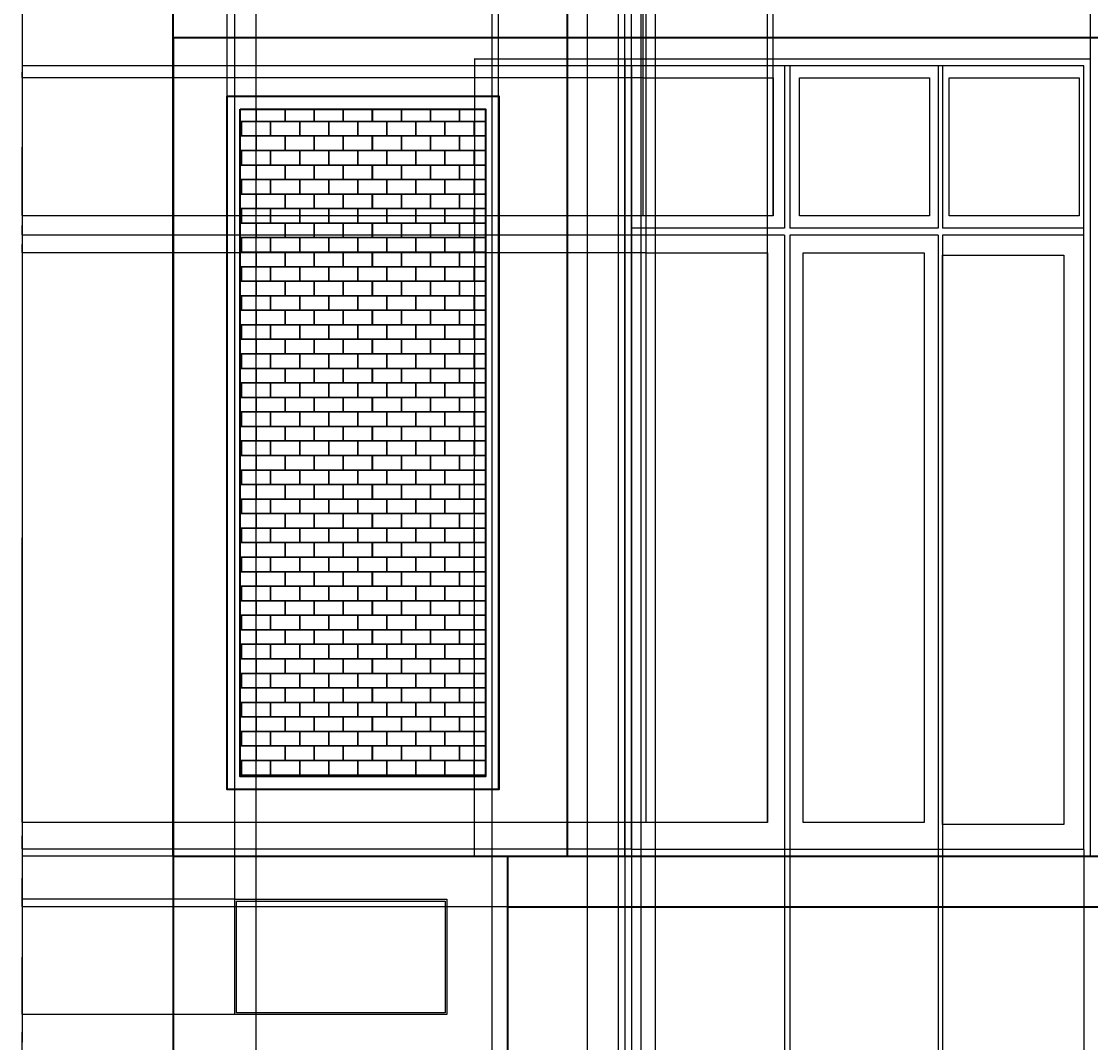
# Model space of a CAD drawing. Units: inches. Extents: x 1231 to 2151, y 481 to 2277.
# Tile 5 of 7: x 1231 to 1819, y 1373 to 1935. Entities that reach past the tile are written whole.
import ezdxf

# ---------------------------------------------------------------- set-up
doc = ezdxf.new("R2010")
doc.units = ezdxf.units.IN
doc.header["$MEASUREMENT"] = 0
for name, color, linetype, lineweight in [('A-ANNO-DIMS', 2, 'Continuous', 18), ('A-DOOR', 4, 'Continuous', 25), ('A-ELEV', 7, 'Continuous', 35), ('A-GLAZ', 3, 'Continuous', 25), ('A-WALL-PATT', 8, 'Continuous', 13)]:
    doc.layers.add(name, color=color, linetype=linetype, lineweight=lineweight)
doc.styles.get("Standard").update_dxf_attribs({"font": 'arial.ttf'})
doc.dimstyles.get("Standard").update_dxf_attribs({"dimtxt": 0.18, "dimasz": 0.18, "dimexe": 0.18, "dimexo": 0.0625, "dimgap": 0.09, "dimtad": 0, "dimtih": 1, "dimtoh": 1, "dimdec": 0, "dimzin": 0, "dimdsep": 46, "dimlunit": 3, "dimtxsty": 'Standard', "dimcen": 0.09, "dimadec": 0, "dimazin": 0, "dimtfac": 1, "dimtdec": 0, "dimtofl": 0, "dimtmove": 0, "dimatfit": 3, "dimfxl": 1, "dimtolj": 1, "dimtzin": 0, "dimarcsym": 0})

# ---------------------------------------------------------------- blocks, each defined once
blk = doc.blocks.new('*D2')
at = {"layer": 'A-ANNO-DIMS', "color": 0, "lineweight": -2, "transparency": 16777216}
for p, q in [((1314.18, 2193.78), (1230.78, 2193.78)), ((1230.96, 2193.6), (1230.96, 1378.92)), ((1230.96, 563.87), (1230.96, 1378.55)), ((1314.18, 563.69), (1230.78, 563.69))]:
    blk.add_line(p, q, dxfattribs=at)
at = {"layer": 'A-ANNO-DIMS', "color": 0, "transparency": 16777216}
for points in [[(1230.93, 2193.6), (1230.99, 2193.6), (1230.96, 2193.78)], [(1230.93, 563.87), (1230.99, 563.87), (1230.96, 563.69)]]:
    blk.add_solid(points, dxfattribs=at)
at = {"layer": 'Defpoints', "color": 0, "transparency": 16777216}
for p in [(1230.96, 2193.78), (1314.24, 2193.78), (1314.24, 563.69)]:
    blk.add_point(p, dxfattribs=at)
at = {"layer": 'A-ANNO-DIMS', "color": 0, "transparency": 16777216, "insert": (1230.96, 1378.74), "char_height": 0.18, "attachment_point": 5}
blk.add_mtext('\\A1;1630', dxfattribs=at)
blk = doc.blocks.new('*D15')
at = {"layer": 'A-ANNO-DIMS', "color": 0, "lineweight": -2, "transparency": 16777216}
for p, q in [((1314.24, 1475.61), (1314.24, 2276.71)), ((1314.42, 2276.53), (1328.56, 2276.53)), ((1343.64, 2276.53), (1329.49, 2276.53)), ((1343.82, 1512.24), (1343.82, 2276.71))]:
    blk.add_line(p, q, dxfattribs=at)
at = {"layer": 'A-ANNO-DIMS', "color": 0, "transparency": 16777216}
for points in [[(1314.42, 2276.56), (1314.42, 2276.5), (1314.24, 2276.53)], [(1343.64, 2276.56), (1343.64, 2276.5), (1343.82, 2276.53)]]:
    blk.add_solid(points, dxfattribs=at)
at = {"layer": 'Defpoints', "color": 0, "transparency": 16777216}
for p in [(1343.82, 2276.53), (1343.82, 1512.17), (1314.24, 1475.54)]:
    blk.add_point(p, dxfattribs=at)
at = {"layer": 'A-ANNO-DIMS', "color": 0, "transparency": 16777216, "insert": (1329.03, 2276.53), "char_height": 0.18, "attachment_point": 5}
blk.add_mtext('\\A1;29.575', dxfattribs=at)
blk = doc.blocks.new('*D16')
at = {"layer": 'A-ANNO-DIMS', "color": 0, "lineweight": -2, "transparency": 16777216}
for p, q in [((1343.82, 1512.24), (1343.82, 2276.71)), ((1344, 2276.53), (1418.14, 2276.53)), ((1493.2, 2276.53), (1419.06, 2276.53)), ((1493.38, 1512.24), (1493.38, 2276.71))]:
    blk.add_line(p, q, dxfattribs=at)
at = {"layer": 'A-ANNO-DIMS', "color": 0, "transparency": 16777216}
for points in [[(1344, 2276.56), (1344, 2276.5), (1343.82, 2276.53)], [(1493.2, 2276.56), (1493.2, 2276.5), (1493.38, 2276.53)]]:
    blk.add_solid(points, dxfattribs=at)
at = {"layer": 'Defpoints', "color": 0, "transparency": 16777216}
for p in [(1493.38, 2276.53), (1343.82, 1512.17), (1493.38, 1512.17)]:
    blk.add_point(p, dxfattribs=at)
at = {"layer": 'A-ANNO-DIMS', "color": 0, "transparency": 16777216, "insert": (1418.6, 2276.53), "char_height": 0.18, "attachment_point": 5}
blk.add_mtext('\\A1;149.57', dxfattribs=at)
blk = doc.blocks.new('*D17')
at = {"layer": 'A-ANNO-DIMS', "color": 0, "lineweight": -2, "transparency": 16777216}
for p, q in [((1493.38, 1512.24), (1493.38, 2276.71)), ((1493.56, 2276.53), (1527.71, 2276.53)), ((1562.61, 2276.53), (1528.46, 2276.53)), ((1562.79, 1475.61), (1562.79, 2276.71))]:
    blk.add_line(p, q, dxfattribs=at)
at = {"layer": 'A-ANNO-DIMS', "color": 0, "transparency": 16777216}
for points in [[(1493.56, 2276.56), (1493.56, 2276.5), (1493.38, 2276.53)], [(1562.61, 2276.56), (1562.61, 2276.5), (1562.79, 2276.53)]]:
    blk.add_solid(points, dxfattribs=at)
at = {"layer": 'Defpoints', "color": 0, "transparency": 16777216}
for p in [(1562.79, 2276.53), (1493.38, 1512.17), (1562.79, 1475.54)]:
    blk.add_point(p, dxfattribs=at)
at = {"layer": 'A-ANNO-DIMS', "color": 0, "transparency": 16777216, "insert": (1528.09, 2276.53), "char_height": 0.18, "attachment_point": 5}
blk.add_mtext('\\A1;69.41', dxfattribs=at)
blk = doc.blocks.new('*D18')
at = {"layer": 'A-ANNO-DIMS', "color": 0, "lineweight": -2, "transparency": 16777216}
for p, q in [((1562.79, 1914.62), (1562.79, 2276.71)), ((1562.97, 2276.53), (1690.65, 2276.53)), ((1819.13, 2276.53), (1691.45, 2276.53)), ((1819.31, 1914.62), (1819.31, 2276.71))]:
    blk.add_line(p, q, dxfattribs=at)
at = {"layer": 'A-ANNO-DIMS', "color": 0, "transparency": 16777216}
for points in [[(1562.97, 2276.56), (1562.97, 2276.5), (1562.79, 2276.53)], [(1819.13, 2276.56), (1819.13, 2276.5), (1819.31, 2276.53)]]:
    blk.add_solid(points, dxfattribs=at)
at = {"layer": 'Defpoints', "color": 0, "transparency": 16777216}
for p in [(1819.31, 2276.53), (1562.79, 1914.56), (1819.31, 1914.56)]:
    blk.add_point(p, dxfattribs=at)
at = {"layer": 'A-ANNO-DIMS', "color": 0, "transparency": 16777216, "insert": (1691.05, 2276.53), "char_height": 0.18, "attachment_point": 5}
blk.add_mtext('\\A1;256.5', dxfattribs=at)
blk = doc.blocks.new('*D32')
at = {"layer": 'A-ANNO-DIMS', "color": 0, "lineweight": -2, "transparency": 16777216}
for p, q in [((1314.24, 1043.75), (1314.24, 2276.71)), ((1314.42, 2276.53), (1336.68, 2276.53)), ((1359.73, 2276.53), (1337.47, 2276.53)), ((1359.91, 1037.75), (1359.91, 2276.71))]:
    blk.add_line(p, q, dxfattribs=at)
at = {"layer": 'A-ANNO-DIMS', "color": 0, "transparency": 16777216}
for points in [[(1314.42, 2276.56), (1314.42, 2276.5), (1314.24, 2276.53)], [(1359.73, 2276.56), (1359.73, 2276.5), (1359.91, 2276.53)]]:
    blk.add_solid(points, dxfattribs=at)
at = {"layer": 'Defpoints', "color": 0, "transparency": 16777216}
for p in [(1359.91, 2276.53), (1314.24, 1043.69), (1359.91, 1037.69)]:
    blk.add_point(p, dxfattribs=at)
at = {"layer": 'A-ANNO-DIMS', "color": 0, "transparency": 16777216, "insert": (1337.07, 2276.53), "char_height": 0.18, "attachment_point": 5}
blk.add_mtext('\\A1;45.67', dxfattribs=at)
blk = doc.blocks.new('*D33')
at = {"layer": 'A-ANNO-DIMS', "color": 0, "lineweight": -2, "transparency": 16777216}
for p, q in [((1359.91, 1037.75), (1359.91, 2276.71)), ((1360.09, 2276.53), (1424.43, 2276.53)), ((1489.68, 2276.53), (1425.34, 2276.53)), ((1489.86, 1037.75), (1489.86, 2276.71))]:
    blk.add_line(p, q, dxfattribs=at)
at = {"layer": 'A-ANNO-DIMS', "color": 0, "transparency": 16777216}
for points in [[(1360.09, 2276.56), (1360.09, 2276.5), (1359.91, 2276.53)], [(1489.68, 2276.56), (1489.68, 2276.5), (1489.86, 2276.53)]]:
    blk.add_solid(points, dxfattribs=at)
at = {"layer": 'Defpoints', "color": 0, "transparency": 16777216}
for p in [(1489.86, 2276.53), (1359.91, 1037.69), (1489.86, 1037.69)]:
    blk.add_point(p, dxfattribs=at)
at = {"layer": 'A-ANNO-DIMS', "color": 0, "transparency": 16777216, "insert": (1424.88, 2276.53), "char_height": 0.18, "attachment_point": 5}
blk.add_mtext('\\A1;129.95', dxfattribs=at)
blk = doc.blocks.new('*D34')
at = {"layer": 'A-ANNO-DIMS', "color": 0, "lineweight": -2, "transparency": 16777216}
for p, q in [((1489.86, 1037.75), (1489.86, 2276.71)), ((1490.04, 2276.53), (1515.72, 2276.53)), ((1542.2, 2276.53), (1516.51, 2276.53)), ((1542.38, 1043.75), (1542.38, 2276.71))]:
    blk.add_line(p, q, dxfattribs=at)
at = {"layer": 'A-ANNO-DIMS', "color": 0, "transparency": 16777216}
for points in [[(1490.04, 2276.56), (1490.04, 2276.5), (1489.86, 2276.53)], [(1542.2, 2276.56), (1542.2, 2276.5), (1542.38, 2276.53)]]:
    blk.add_solid(points, dxfattribs=at)
at = {"layer": 'Defpoints', "color": 0, "transparency": 16777216}
for p in [(1542.38, 2276.53), (1542.38, 1043.69), (1489.86, 1037.69)]:
    blk.add_point(p, dxfattribs=at)
at = {"layer": 'A-ANNO-DIMS', "color": 0, "transparency": 16777216, "insert": (1516.12, 2276.53), "char_height": 0.18, "attachment_point": 5}
blk.add_mtext('\\A1;52.52', dxfattribs=at)
blk = doc.blocks.new('*D35')
at = {"layer": 'A-ANNO-DIMS', "color": 0, "lineweight": -2, "transparency": 16777216}
for p, q in [((1542.38, 1043.75), (1542.38, 2276.71)), ((1542.56, 2276.53), (1556.6, 2276.53)), ((1571.58, 2276.53), (1557.53, 2276.53)), ((1571.76, 1043.75), (1571.76, 2276.71))]:
    blk.add_line(p, q, dxfattribs=at)
at = {"layer": 'A-ANNO-DIMS', "color": 0, "transparency": 16777216}
for points in [[(1542.56, 2276.56), (1542.56, 2276.5), (1542.38, 2276.53)], [(1571.58, 2276.56), (1571.58, 2276.5), (1571.76, 2276.53)]]:
    blk.add_solid(points, dxfattribs=at)
at = {"layer": 'Defpoints', "color": 0, "transparency": 16777216}
for p in [(1571.76, 2276.53), (1542.38, 1043.69), (1571.76, 1043.69)]:
    blk.add_point(p, dxfattribs=at)
at = {"layer": 'A-ANNO-DIMS', "color": 0, "transparency": 16777216, "insert": (1557.07, 2276.53), "char_height": 0.18, "attachment_point": 5}
blk.add_mtext('\\A1;29.385', dxfattribs=at)
blk = doc.blocks.new('*D36')
at = {"layer": 'A-ANNO-DIMS', "color": 0, "lineweight": -2, "transparency": 16777216}
for p, q in [((1571.76, 1043.75), (1571.76, 2276.71)), ((1571.94, 2276.53), (1575.38, 2276.53)), ((1579.61, 2276.53), (1576.17, 2276.53)), ((1579.79, 1032.87), (1579.79, 2276.71))]:
    blk.add_line(p, q, dxfattribs=at)
at = {"layer": 'A-ANNO-DIMS', "color": 0, "transparency": 16777216}
for points in [[(1571.94, 2276.56), (1571.94, 2276.5), (1571.76, 2276.53)], [(1579.61, 2276.56), (1579.61, 2276.5), (1579.79, 2276.53)]]:
    blk.add_solid(points, dxfattribs=at)
at = {"layer": 'Defpoints', "color": 0, "transparency": 16777216}
for p in [(1579.79, 2276.53), (1571.76, 1043.69), (1579.79, 1032.81)]:
    blk.add_point(p, dxfattribs=at)
at = {"layer": 'A-ANNO-DIMS', "color": 0, "transparency": 16777216, "insert": (1575.78, 2276.53), "char_height": 0.18, "attachment_point": 5}
blk.add_mtext('\\A1;8.033', dxfattribs=at)
blk = doc.blocks.new('*D50')
at = {"layer": 'A-ANNO-DIMS', "color": 0, "lineweight": -2, "transparency": 16777216}
for p, q in [((1542.38, 563.75), (1542.38, 2276.71)), ((1542.56, 2276.53), (1550.52, 2276.53)), ((1559.26, 2276.53), (1551.3, 2276.53)), ((1559.44, 576.65), (1559.44, 2276.71))]:
    blk.add_line(p, q, dxfattribs=at)
at = {"layer": 'A-ANNO-DIMS', "color": 0, "transparency": 16777216}
for points in [[(1542.56, 2276.56), (1542.56, 2276.5), (1542.38, 2276.53)], [(1559.26, 2276.56), (1559.26, 2276.5), (1559.44, 2276.53)]]:
    blk.add_solid(points, dxfattribs=at)
at = {"layer": 'Defpoints', "color": 0, "transparency": 16777216}
for p in [(1559.44, 2276.53), (1559.44, 576.59), (1542.38, 563.69)]:
    blk.add_point(p, dxfattribs=at)
at = {"layer": 'A-ANNO-DIMS', "color": 0, "transparency": 16777216, "insert": (1550.91, 2276.53), "char_height": 0.18, "attachment_point": 5}
blk.add_mtext('\\A1;17.07', dxfattribs=at)
blk = doc.blocks.new('*D58')
at = {"layer": 'A-ANNO-DIMS', "color": 0, "lineweight": -2, "transparency": 16777216}
for p, q in [((1314.24, 1475.61), (1314.24, 2276.71)), ((1314.42, 2276.53), (1330.74, 2276.53)), ((1347.85, 2276.53), (1331.53, 2276.53)), ((1348.03, 1451.84), (1348.03, 2276.71))]:
    blk.add_line(p, q, dxfattribs=at)
at = {"layer": 'A-ANNO-DIMS', "color": 0, "transparency": 16777216}
for points in [[(1314.42, 2276.56), (1314.42, 2276.5), (1314.24, 2276.53)], [(1347.85, 2276.56), (1347.85, 2276.5), (1348.03, 2276.53)]]:
    blk.add_solid(points, dxfattribs=at)
at = {"layer": 'Defpoints', "color": 0, "transparency": 16777216}
for p in [(1348.03, 2276.53), (1314.24, 1475.54), (1348.03, 1451.77)]:
    blk.add_point(p, dxfattribs=at)
at = {"layer": 'A-ANNO-DIMS', "color": 0, "transparency": 16777216, "insert": (1331.14, 2276.53), "char_height": 0.18, "attachment_point": 5}
blk.add_mtext('\\A1;33.79', dxfattribs=at)
blk = doc.blocks.new('*D59')
at = {"layer": 'A-ANNO-DIMS', "color": 0, "lineweight": -2, "transparency": 16777216}
for p, q in [((1314.18, 1475.54), (1230.78, 1475.54)), ((1230.96, 1475.36), (1230.96, 1463.84)), ((1230.96, 1451.95), (1230.96, 1463.48)), ((1347.97, 1451.77), (1230.78, 1451.77))]:
    blk.add_line(p, q, dxfattribs=at)
at = {"layer": 'A-ANNO-DIMS', "color": 0, "transparency": 16777216}
for points in [[(1230.93, 1475.36), (1230.99, 1475.36), (1230.96, 1475.54)], [(1230.93, 1451.95), (1230.99, 1451.95), (1230.96, 1451.77)]]:
    blk.add_solid(points, dxfattribs=at)
at = {"layer": 'Defpoints', "color": 0, "transparency": 16777216}
for p in [(1314.24, 1475.54), (1230.96, 1451.77), (1348.03, 1451.77)]:
    blk.add_point(p, dxfattribs=at)
at = {"layer": 'A-ANNO-DIMS', "color": 0, "transparency": 16777216, "insert": (1230.96, 1463.66), "char_height": 0.18, "attachment_point": 5}
blk.add_mtext('\\A1;23.77', dxfattribs=at)
blk = doc.blocks.new('*D60')
at = {"layer": 'A-ANNO-DIMS', "color": 0, "lineweight": -2, "transparency": 16777216}
for p, q in [((1347.97, 1451.77), (1230.78, 1451.77)), ((1230.96, 1451.59), (1230.96, 1420.21)), ((1230.96, 1388.46), (1230.96, 1419.84)), ((1347.97, 1388.28), (1230.78, 1388.28))]:
    blk.add_line(p, q, dxfattribs=at)
at = {"layer": 'A-ANNO-DIMS', "color": 0, "transparency": 16777216}
for points in [[(1230.93, 1451.59), (1230.99, 1451.59), (1230.96, 1451.77)], [(1230.93, 1388.46), (1230.99, 1388.46), (1230.96, 1388.28)]]:
    blk.add_solid(points, dxfattribs=at)
at = {"layer": 'Defpoints', "color": 0, "transparency": 16777216}
for p in [(1348.03, 1451.77), (1230.96, 1388.28), (1348.03, 1388.28)]:
    blk.add_point(p, dxfattribs=at)
at = {"layer": 'A-ANNO-DIMS', "color": 0, "transparency": 16777216, "insert": (1230.96, 1420.03), "char_height": 0.18, "attachment_point": 5}
blk.add_mtext('\\A1;63.5', dxfattribs=at)
blk = doc.blocks.new('*D61')
at = {"layer": 'A-ANNO-DIMS', "color": 0, "lineweight": -2, "transparency": 16777216}
for p, q in [((1347.97, 1388.28), (1230.78, 1388.28)), ((1230.96, 1388.1), (1230.96, 1372.98)), ((1230.96, 1357.51), (1230.96, 1372.62)), ((1347.97, 1357.33), (1230.78, 1357.33))]:
    blk.add_line(p, q, dxfattribs=at)
at = {"layer": 'A-ANNO-DIMS', "color": 0, "transparency": 16777216}
for points in [[(1230.93, 1388.1), (1230.99, 1388.1), (1230.96, 1388.28)], [(1230.93, 1357.51), (1230.99, 1357.51), (1230.96, 1357.33)]]:
    blk.add_solid(points, dxfattribs=at)
at = {"layer": 'Defpoints', "color": 0, "transparency": 16777216}
for p in [(1348.03, 1388.28), (1230.96, 1357.33), (1348.03, 1357.33)]:
    blk.add_point(p, dxfattribs=at)
at = {"layer": 'A-ANNO-DIMS', "color": 0, "transparency": 16777216, "insert": (1230.96, 1372.8), "char_height": 0.18, "attachment_point": 5}
blk.add_mtext('\\A1;30.954', dxfattribs=at)
blk = doc.blocks.new('*D67')
at = {"layer": 'A-ANNO-DIMS', "color": 0, "lineweight": -2, "transparency": 16777216}
for p, q in [((1498.25, 1475.54), (1230.78, 1475.54)), ((1230.96, 1475.36), (1230.96, 1461.72)), ((1230.96, 1447.72), (1230.96, 1461.36)), ((1498.25, 1447.54), (1230.78, 1447.54))]:
    blk.add_line(p, q, dxfattribs=at)
at = {"layer": 'A-ANNO-DIMS', "color": 0, "transparency": 16777216}
for points in [[(1230.93, 1475.36), (1230.99, 1475.36), (1230.96, 1475.54)], [(1230.93, 1447.72), (1230.99, 1447.72), (1230.96, 1447.54)]]:
    blk.add_solid(points, dxfattribs=at)
at = {"layer": 'Defpoints', "color": 0, "transparency": 16777216}
for p in [(1230.96, 1475.54), (1498.31, 1475.54), (1498.31, 1447.54)]:
    blk.add_point(p, dxfattribs=at)
at = {"layer": 'A-ANNO-DIMS', "color": 0, "transparency": 16777216, "insert": (1230.96, 1461.54), "char_height": 0.18, "attachment_point": 5}
blk.add_mtext('\\A1;28.005', dxfattribs=at)
blk = doc.blocks.new('*D83')
at = {"layer": 'A-ANNO-DIMS', "color": 0, "lineweight": -2, "transparency": 16777216}
for p, q in [((1562.73, 1914.56), (1479.86, 1914.56)), ((1480.04, 1914.38), (1480.04, 1695.23)), ((1480.04, 1475.72), (1480.04, 1694.87)), ((1562.73, 1475.54), (1479.86, 1475.54))]:
    blk.add_line(p, q, dxfattribs=at)
at = {"layer": 'A-ANNO-DIMS', "color": 0, "transparency": 16777216}
for points in [[(1480.01, 1914.38), (1480.07, 1914.38), (1480.04, 1914.56)], [(1480.01, 1475.72), (1480.07, 1475.72), (1480.04, 1475.54)]]:
    blk.add_solid(points, dxfattribs=at)
at = {"layer": 'Defpoints', "color": 0, "transparency": 16777216}
for p in [(1480.04, 1914.56), (1562.79, 1914.56), (1562.79, 1475.54)]:
    blk.add_point(p, dxfattribs=at)
at = {"layer": 'A-ANNO-DIMS', "color": 0, "transparency": 16777216, "insert": (1480.04, 1695.05), "char_height": 0.18, "attachment_point": 5}
blk.add_mtext('\\A1;439', dxfattribs=at)
blk = doc.blocks.new('*D84')
at = {"layer": 'A-ANNO-DIMS', "color": 0, "lineweight": -2, "transparency": 16777216}
for p, q in [((1574.54, 1494.13), (1230.78, 1494.13)), ((1230.96, 1493.95), (1230.96, 1486.91)), ((1230.96, 1479.5), (1230.96, 1486.54)), ((1566.5, 1479.32), (1230.78, 1479.32))]:
    blk.add_line(p, q, dxfattribs=at)
at = {"layer": 'A-ANNO-DIMS', "color": 0, "transparency": 16777216}
for points in [[(1230.93, 1493.95), (1230.99, 1493.95), (1230.96, 1494.13)], [(1230.93, 1479.5), (1230.99, 1479.5), (1230.96, 1479.32)]]:
    blk.add_solid(points, dxfattribs=at)
at = {"layer": 'Defpoints', "color": 0, "transparency": 16777216}
for p in [(1230.96, 1494.13), (1574.6, 1494.13), (1566.56, 1479.32)]:
    blk.add_point(p, dxfattribs=at)
at = {"layer": 'A-ANNO-DIMS', "color": 0, "transparency": 16777216, "insert": (1230.96, 1486.72), "char_height": 0.18, "attachment_point": 5}
blk.add_mtext('\\A1;14.818', dxfattribs=at)
blk = doc.blocks.new('*D85')
at = {"layer": 'A-ANNO-DIMS', "color": 0, "lineweight": -2, "transparency": 16777216}
for p, q in [((1574.54, 1807.75), (1230.78, 1807.75)), ((1230.96, 1807.57), (1230.96, 1651.12)), ((1230.96, 1494.31), (1230.96, 1650.76)), ((1574.54, 1494.13), (1230.78, 1494.13))]:
    blk.add_line(p, q, dxfattribs=at)
at = {"layer": 'A-ANNO-DIMS', "color": 0, "transparency": 16777216}
for points in [[(1230.93, 1807.57), (1230.99, 1807.57), (1230.96, 1807.75)], [(1230.93, 1494.31), (1230.99, 1494.31), (1230.96, 1494.13)]]:
    blk.add_solid(points, dxfattribs=at)
at = {"layer": 'Defpoints', "color": 0, "transparency": 16777216}
for p in [(1230.96, 1807.75), (1574.6, 1807.75), (1574.6, 1494.13)]:
    blk.add_point(p, dxfattribs=at)
at = {"layer": 'A-ANNO-DIMS', "color": 0, "transparency": 16777216, "insert": (1230.96, 1650.94), "char_height": 0.18, "attachment_point": 5}
blk.add_mtext('\\A1;313.6', dxfattribs=at)
blk = doc.blocks.new('*D86')
at = {"layer": 'A-ANNO-DIMS', "color": 0, "lineweight": -2, "transparency": 16777216}
for p, q in [((1566.5, 1817.51), (1230.78, 1817.51)), ((1230.96, 1817.33), (1230.96, 1812.81)), ((1574.54, 1807.75), (1230.78, 1807.75)), ((1230.96, 1807.93), (1230.96, 1812.45))]:
    blk.add_line(p, q, dxfattribs=at)
at = {"layer": 'A-ANNO-DIMS', "color": 0, "transparency": 16777216}
for points in [[(1230.93, 1817.33), (1230.99, 1817.33), (1230.96, 1817.51)], [(1230.93, 1807.93), (1230.99, 1807.93), (1230.96, 1807.75)]]:
    blk.add_solid(points, dxfattribs=at)
at = {"layer": 'Defpoints', "color": 0, "transparency": 16777216}
for p in [(1230.96, 1817.51), (1566.56, 1817.51), (1574.6, 1807.75)]:
    blk.add_point(p, dxfattribs=at)
at = {"layer": 'A-ANNO-DIMS', "color": 0, "transparency": 16777216, "insert": (1230.96, 1812.63), "char_height": 0.18, "attachment_point": 5}
blk.add_mtext('\\A1;9.758', dxfattribs=at)
blk = doc.blocks.new('*D87')
at = {"layer": 'A-ANNO-DIMS', "color": 0, "lineweight": -2, "transparency": 16777216}
for p, q in [((1572.8, 1828.25), (1230.78, 1828.25)), ((1230.96, 1828.07), (1230.96, 1823.06)), ((1230.96, 1817.69), (1230.96, 1822.7)), ((1566.5, 1817.51), (1230.78, 1817.51))]:
    blk.add_line(p, q, dxfattribs=at)
at = {"layer": 'A-ANNO-DIMS', "color": 0, "transparency": 16777216}
for points in [[(1230.93, 1828.07), (1230.99, 1828.07), (1230.96, 1828.25)], [(1230.93, 1817.69), (1230.99, 1817.69), (1230.96, 1817.51)]]:
    blk.add_solid(points, dxfattribs=at)
at = {"layer": 'Defpoints', "color": 0, "transparency": 16777216}
for p in [(1230.96, 1828.25), (1572.87, 1828.25), (1566.56, 1817.51)]:
    blk.add_point(p, dxfattribs=at)
at = {"layer": 'A-ANNO-DIMS', "color": 0, "transparency": 16777216, "insert": (1230.96, 1822.88), "char_height": 0.18, "attachment_point": 5}
blk.add_mtext('\\A1;10.739', dxfattribs=at)
blk = doc.blocks.new('*D88')
at = {"layer": 'A-ANNO-DIMS', "color": 0, "lineweight": -2, "transparency": 16777216}
for p, q in [((1572.8, 1904.15), (1230.78, 1904.15)), ((1230.96, 1903.97), (1230.96, 1866.38)), ((1230.96, 1828.43), (1230.96, 1866.02)), ((1572.8, 1828.25), (1230.78, 1828.25))]:
    blk.add_line(p, q, dxfattribs=at)
at = {"layer": 'A-ANNO-DIMS', "color": 0, "transparency": 16777216}
for points in [[(1230.93, 1903.97), (1230.99, 1903.97), (1230.96, 1904.15)], [(1230.93, 1828.43), (1230.99, 1828.43), (1230.96, 1828.25)]]:
    blk.add_solid(points, dxfattribs=at)
at = {"layer": 'Defpoints', "color": 0, "transparency": 16777216}
for p in [(1230.96, 1904.15), (1572.87, 1904.15), (1572.87, 1828.25)]:
    blk.add_point(p, dxfattribs=at)
at = {"layer": 'A-ANNO-DIMS', "color": 0, "transparency": 16777216, "insert": (1230.96, 1866.2), "char_height": 0.18, "attachment_point": 5}
blk.add_mtext('\\A1;75.9', dxfattribs=at)
blk = doc.blocks.new('*D89')
at = {"layer": 'A-ANNO-DIMS', "color": 0, "lineweight": -2, "transparency": 16777216}
for p, q in [((1566.5, 1910.79), (1230.78, 1910.79)), ((1230.96, 1910.61), (1230.96, 1907.65)), ((1572.8, 1904.15), (1230.78, 1904.15)), ((1230.96, 1904.33), (1230.96, 1907.28))]:
    blk.add_line(p, q, dxfattribs=at)
at = {"layer": 'A-ANNO-DIMS', "color": 0, "transparency": 16777216}
for points in [[(1230.93, 1910.61), (1230.99, 1910.61), (1230.96, 1910.79)], [(1230.93, 1904.33), (1230.99, 1904.33), (1230.96, 1904.15)]]:
    blk.add_solid(points, dxfattribs=at)
at = {"layer": 'Defpoints', "color": 0, "transparency": 16777216}
for p in [(1230.96, 1910.79), (1566.56, 1910.79), (1572.87, 1904.15)]:
    blk.add_point(p, dxfattribs=at)
at = {"layer": 'A-ANNO-DIMS', "color": 0, "transparency": 16777216, "insert": (1230.96, 1907.47), "char_height": 0.18, "attachment_point": 5}
blk.add_mtext('\\A1;6.64', dxfattribs=at)
blk = doc.blocks.new('*D90')
at = {"layer": 'A-ANNO-DIMS', "color": 0, "lineweight": -2, "transparency": 16777216}
for p, q in [((1566.56, 1479.25), (1566.56, 480.76)), ((1562.79, 1475.48), (1562.79, 480.76)), ((1562.97, 480.94), (1564.3, 480.94)), ((1566.38, 480.94), (1565.05, 480.94))]:
    blk.add_line(p, q, dxfattribs=at)
at = {"layer": 'A-ANNO-DIMS', "color": 0, "transparency": 16777216}
for points in [[(1562.97, 480.97), (1562.97, 480.91), (1562.79, 480.94)], [(1566.38, 480.97), (1566.38, 480.91), (1566.56, 480.94)]]:
    blk.add_solid(points, dxfattribs=at)
at = {"layer": 'Defpoints', "color": 0, "transparency": 16777216}
for p in [(1566.56, 1479.32), (1562.79, 1475.54), (1566.56, 480.94)]:
    blk.add_point(p, dxfattribs=at)
at = {"layer": 'A-ANNO-DIMS', "color": 0, "transparency": 16777216, "insert": (1564.68, 480.94), "char_height": 0.18, "attachment_point": 5}
blk.add_mtext('\\A1;3.771', dxfattribs=at)
blk = doc.blocks.new('*D91')
at = {"layer": 'A-ANNO-DIMS', "color": 0, "lineweight": -2, "transparency": 16777216}
for p, q in [((1566.56, 1479.25), (1566.56, 480.76)), ((1650.77, 1479.25), (1650.77, 480.76)), ((1566.74, 480.94), (1608.34, 480.94)), ((1650.59, 480.94), (1608.99, 480.94))]:
    blk.add_line(p, q, dxfattribs=at)
at = {"layer": 'A-ANNO-DIMS', "color": 0, "transparency": 16777216}
for points in [[(1566.74, 480.97), (1566.74, 480.91), (1566.56, 480.94)], [(1650.59, 480.97), (1650.59, 480.91), (1650.77, 480.94)]]:
    blk.add_solid(points, dxfattribs=at)
at = {"layer": 'Defpoints', "color": 0, "transparency": 16777216}
for p in [(1566.56, 1479.32), (1650.77, 1479.32), (1650.77, 480.94)]:
    blk.add_point(p, dxfattribs=at)
at = {"layer": 'A-ANNO-DIMS', "color": 0, "transparency": 16777216, "insert": (1608.66, 480.94), "char_height": 0.18, "attachment_point": 5}
blk.add_mtext('\\A1;84.2', dxfattribs=at)
blk = doc.blocks.new('*D92')
at = {"layer": 'A-ANNO-DIMS', "color": 0, "lineweight": -2, "transparency": 16777216}
for p, q in [((1653.67, 1479.25), (1653.67, 480.76)), ((1735.42, 1479.25), (1735.42, 480.76)), ((1653.85, 480.94), (1694.15, 480.94)), ((1735.24, 480.94), (1694.94, 480.94))]:
    blk.add_line(p, q, dxfattribs=at)
at = {"layer": 'A-ANNO-DIMS', "color": 0, "transparency": 16777216}
for points in [[(1653.85, 480.97), (1653.85, 480.91), (1653.67, 480.94)], [(1735.24, 480.97), (1735.24, 480.91), (1735.42, 480.94)]]:
    blk.add_solid(points, dxfattribs=at)
at = {"layer": 'Defpoints', "color": 0, "transparency": 16777216}
for p in [(1653.67, 1479.32), (1735.42, 1479.32), (1735.42, 480.94)]:
    blk.add_point(p, dxfattribs=at)
at = {"layer": 'A-ANNO-DIMS', "color": 0, "transparency": 16777216, "insert": (1694.55, 480.94), "char_height": 0.18, "attachment_point": 5}
blk.add_mtext('\\A1;81.75', dxfattribs=at)
blk = doc.blocks.new('*D93')
at = {"layer": 'A-ANNO-DIMS', "color": 0, "lineweight": -2, "transparency": 16777216}
for p, q in [((1737.75, 1479.25), (1737.75, 480.76)), ((1815.54, 1479.25), (1815.54, 480.76)), ((1737.93, 480.94), (1776.25, 480.94)), ((1815.36, 480.94), (1777.04, 480.94))]:
    blk.add_line(p, q, dxfattribs=at)
at = {"layer": 'A-ANNO-DIMS', "color": 0, "transparency": 16777216}
for points in [[(1737.93, 480.97), (1737.93, 480.91), (1737.75, 480.94)], [(1815.36, 480.97), (1815.36, 480.91), (1815.54, 480.94)]]:
    blk.add_solid(points, dxfattribs=at)
at = {"layer": 'Defpoints', "color": 0, "transparency": 16777216}
for p in [(1737.75, 1479.32), (1815.54, 1479.32), (1815.54, 480.94)]:
    blk.add_point(p, dxfattribs=at)
at = {"layer": 'A-ANNO-DIMS', "color": 0, "transparency": 16777216, "insert": (1776.64, 480.94), "char_height": 0.18, "attachment_point": 5}
blk.add_mtext('\\A1;77.79', dxfattribs=at)
blk = doc.blocks.new('*D94')
at = {"layer": 'A-ANNO-DIMS', "color": 0, "lineweight": -2, "transparency": 16777216}
for p, q in [((1566.56, 1479.38), (1566.56, 2276.71)), ((1566.74, 2276.53), (1570.19, 2276.53)), ((1574.42, 2276.53), (1570.98, 2276.53)), ((1574.6, 1494.2), (1574.6, 2276.71))]:
    blk.add_line(p, q, dxfattribs=at)
at = {"layer": 'A-ANNO-DIMS', "color": 0, "transparency": 16777216}
for points in [[(1566.74, 2276.56), (1566.74, 2276.5), (1566.56, 2276.53)], [(1574.42, 2276.56), (1574.42, 2276.5), (1574.6, 2276.53)]]:
    blk.add_solid(points, dxfattribs=at)
at = {"layer": 'Defpoints', "color": 0, "transparency": 16777216}
for p in [(1574.6, 2276.53), (1574.6, 1494.13), (1566.56, 1479.32)]:
    blk.add_point(p, dxfattribs=at)
at = {"layer": 'A-ANNO-DIMS', "color": 0, "transparency": 16777216, "insert": (1570.58, 2276.53), "char_height": 0.18, "attachment_point": 5}
blk.add_mtext('\\A1;8.042', dxfattribs=at)
blk = doc.blocks.new('*D95')
at = {"layer": 'A-ANNO-DIMS', "color": 0, "lineweight": -2, "transparency": 16777216}
for p, q in [((1574.6, 1494.2), (1574.6, 2276.71)), ((1574.78, 2276.53), (1607.58, 2276.53)), ((1641.16, 2276.53), (1608.37, 2276.53)), ((1641.34, 1494.2), (1641.34, 2276.71))]:
    blk.add_line(p, q, dxfattribs=at)
at = {"layer": 'A-ANNO-DIMS', "color": 0, "transparency": 16777216}
for points in [[(1574.78, 2276.56), (1574.78, 2276.5), (1574.6, 2276.53)], [(1641.16, 2276.56), (1641.16, 2276.5), (1641.34, 2276.53)]]:
    blk.add_solid(points, dxfattribs=at)
at = {"layer": 'Defpoints', "color": 0, "transparency": 16777216}
for p in [(1641.34, 2276.53), (1574.6, 1494.13), (1641.34, 1494.13)]:
    blk.add_point(p, dxfattribs=at)
at = {"layer": 'A-ANNO-DIMS', "color": 0, "transparency": 16777216, "insert": (1607.97, 2276.53), "char_height": 0.18, "attachment_point": 5}
blk.add_mtext('\\A1;66.74', dxfattribs=at)
blk = doc.blocks.new('*D96')
at = {"layer": 'A-ANNO-DIMS', "color": 0, "lineweight": -2, "transparency": 16777216}
for p, q in [((1572.87, 1828.31), (1572.87, 2276.71)), ((1573.05, 2276.53), (1608.26, 2276.53)), ((1644.26, 2276.53), (1609.05, 2276.53)), ((1644.44, 1828.31), (1644.44, 2276.71))]:
    blk.add_line(p, q, dxfattribs=at)
at = {"layer": 'A-ANNO-DIMS', "color": 0, "transparency": 16777216}
for points in [[(1573.05, 2276.56), (1573.05, 2276.5), (1572.87, 2276.53)], [(1644.26, 2276.56), (1644.26, 2276.5), (1644.44, 2276.53)]]:
    blk.add_solid(points, dxfattribs=at)
at = {"layer": 'Defpoints', "color": 0, "transparency": 16777216}
for p in [(1644.44, 2276.53), (1572.87, 1828.25), (1644.44, 1828.25)]:
    blk.add_point(p, dxfattribs=at)
at = {"layer": 'A-ANNO-DIMS', "color": 0, "transparency": 16777216, "insert": (1608.65, 2276.53), "char_height": 0.18, "attachment_point": 5}
blk.add_mtext('\\A1;71.57', dxfattribs=at)

msp = doc.modelspace()

# ---------------------------------------------------------------- hatches: boundary and pattern name
at = {"layer": 'A-WALL-PATT'}
h = msp.add_hatch(dxfattribs=at)
h.set_pattern_fill('AR-B816C', color=256)
h.paths.add_polyline_path([(1486.2072, 1886.877), (1350.9925, 1886.877), (1350.9925, 1519.3518), (1486.2072, 1519.3518)])

# ---------------------------------------------------------------- linework, layer by layer
at = {"layer": 'A-DOOR'}
for p, q in [((1819.3087, 1914.557), (1562.7916, 1914.557)), ((1562.7916, 1914.557), (1562.7916, 1475.5441)), ((1819.3087, 1475.5441), (1819.3087, 1914.557)), ((1815.5376, 1910.786), (1566.5626, 1910.786)), ((1566.5626, 1910.786), (1566.5626, 1479.3152)), ((1650.766, 1910.786), (1650.766, 1821.4896)), ((1653.6719, 1910.786), (1653.6719, 1821.4896)), ((1735.4237, 1910.786), (1735.4237, 1821.4896)), ((1737.7463, 1910.786), (1737.7463, 1821.4896)), ((1815.5376, 1479.3152), (1815.5376, 1910.786)), ((1650.766, 1821.4896), (1566.5626, 1821.4896)), ((1735.4237, 1821.4896), (1653.6719, 1821.4896)), ((1815.5376, 1821.4896), (1737.7463, 1821.4896)), ((1650.766, 1817.5102), (1566.5626, 1817.5102)), ((1650.766, 1817.5102), (1650.766, 1479.3152)), ((1653.6719, 1817.5102), (1653.6719, 1479.3152)), ((1735.4237, 1817.5102), (1653.6719, 1817.5102)), ((1735.4237, 1817.5102), (1735.4237, 1479.3152)), ((1815.5376, 1817.5102), (1737.7463, 1817.5102)), ((1737.7463, 1817.5102), (1737.7463, 1479.3152)), ((1566.5626, 1479.3152), (1815.5376, 1479.3152)), ((1562.7916, 1475.5441), (1819.3087, 1475.5441))]:
    msp.add_line(p, q, dxfattribs=at)
for points in [[(1572.8669, 1904.1464), (1644.4374, 1904.1464), (1644.4374, 1828.2487), (1572.8669, 1828.2487)], [(1659.0358, 1904.1464), (1730.6063, 1904.1464), (1730.6063, 1828.2487), (1659.0358, 1828.2487)], [(1741.4582, 1904.1464), (1813.0288, 1904.1464), (1813.0288, 1828.2487), (1741.4582, 1828.2487)], [(1574.6049, 1807.7526), (1641.3412, 1807.7526), (1641.3412, 1494.1329), (1574.6049, 1494.1329)], [(1660.9962, 1807.7526), (1727.7324, 1807.7526), (1727.7324, 1494.1329), (1660.9962, 1494.1329)], [(1737.7463, 1806.5252), (1804.4825, 1806.5252), (1804.4825, 1492.9055), (1737.7463, 1492.9055)]]:
    msp.add_lwpolyline(points, close=True, dxfattribs=at)
at = {"layer": 'A-ELEV'}
for p, q in [((1314.2408, 1475.5441), (1314.2408, 2193.7789)), ((1531.2103, 1475.5441), (1531.2103, 1973.8854)), ((2067.6855, 1926.2862), (1314.2408, 1926.2862)), ((1314.2408, 1926.2862), (1314.2408, 563.6912)), ((1314.2408, 1475.5441), (2067.6855, 1475.5441)), ((1498.3132, 1475.5441), (1498.3132, 1170.3351)), ((1498.3132, 1447.5396), (2067.6855, 1447.5396))]:
    msp.add_line(p, q, dxfattribs=at)
for points in [[(1343.8157, 1894.0538), (1493.3841, 1894.0538), (1493.3841, 1512.1749), (1343.8157, 1512.1749)], [(1350.9925, 1886.877), (1486.2072, 1886.877), (1486.2072, 1519.3518), (1350.9925, 1519.3518)]]:
    msp.add_lwpolyline(points, close=True, dxfattribs=at)
at = {"layer": 'A-GLAZ'}
for points in [[(1348.0309, 1451.7741), (1464.8184, 1451.7741), (1464.8184, 1388.2789), (1348.0309, 1388.2789)], [(1348.9993, 1450.8057), (1463.8499, 1450.8057), (1463.8499, 1389.2474), (1348.9993, 1389.2474)]]:
    msp.add_lwpolyline(points, close=True, dxfattribs=at)

# ---------------------------------------------------------------- dimensions: what is measured, and where the dimension line sits
at = {"layer": 'A-ANNO-DIMS'}
for base, p1, p2, override, picture, middle in [((1343.8157, 2276.5289), (1314.2408, 1475.5441), (1343.8157, 1512.1749), {"dimdec": 3, "dimlfac": 1, "dimrnd": 0, "dimzin": 0, "dimdsep": 46, "dimlunit": 2}, '*D15', (1329.0282, 2276.5289)), ((1359.9075, 2276.5289), (1314.2408, 1043.6912), (1359.9075, 1037.6872), {"dimdec": 2, "dimlfac": 1, "dimrnd": 0, "dimzin": 0, "dimdsep": 46, "dimlunit": 2}, '*D32', (1337.0741, 2276.5289)), ((1348.0309, 2276.5289), (1314.2408, 1475.5441), (1348.0309, 1451.7741), {"dimdec": 2, "dimlfac": 1, "dimrnd": 0, "dimzin": 0, "dimdsep": 46, "dimlunit": 2}, '*D58', (1331.1358, 2276.5289)), ((1493.3841, 2276.5289), (1343.8157, 1512.1749), (1493.3841, 1512.1749), {"dimdec": 2, "dimlfac": 1, "dimrnd": 0, "dimzin": 0, "dimdsep": 46, "dimlunit": 2}, '*D16', (1418.5999, 2276.5289)), ((1489.8565, 2276.5289), (1359.9075, 1037.6872), (1489.8565, 1037.6872), {"dimdec": 2, "dimlfac": 1, "dimrnd": 0, "dimzin": 0, "dimdsep": 46, "dimlunit": 2}, '*D33', (1424.882, 2276.5289)), ((1542.3752, 2276.5289), (1489.8565, 1037.6872), (1542.3752, 1043.6912), {"dimdec": 2, "dimlfac": 1, "dimrnd": 0, "dimzin": 0, "dimdsep": 46, "dimlunit": 2}, '*D34', (1516.1158, 2276.5289)), ((1562.7916, 2276.5289), (1493.3841, 1512.1749), (1562.7916, 1475.5441), {"dimdec": 2, "dimlfac": 1, "dimrnd": 0, "dimzin": 0, "dimdsep": 46, "dimlunit": 2}, '*D17', (1528.0878, 2276.5289)), ((1571.76, 2276.5289), (1542.3752, 1043.6912), (1571.76, 1043.6912), {"dimdec": 3, "dimlfac": 1, "dimrnd": 0, "dimzin": 0, "dimdsep": 46, "dimlunit": 2}, '*D35', (1557.0676, 2276.5289)), ((1559.4446, 2276.5289), (1542.3752, 563.6912), (1559.4446, 576.5889), {"dimdec": 2, "dimlfac": 1, "dimrnd": 0, "dimzin": 0, "dimdsep": 46, "dimlunit": 2}, '*D50', (1550.9099, 2276.5289)), ((1819.3087, 2276.5289), (1562.7916, 1914.557), (1819.3087, 1914.557), {"dimdec": 1, "dimlfac": 1, "dimrnd": 0, "dimzin": 0, "dimdsep": 46, "dimlunit": 2}, '*D18', (1691.0501, 2276.5289)), ((1574.6049, 2276.5289), (1566.5626, 1479.3152), (1574.6049, 1494.1329), {"dimdec": 3, "dimlfac": 1, "dimrnd": 0, "dimzin": 0, "dimdsep": 46, "dimlunit": 2}, '*D94', (1570.5838, 2276.5289)), ((1579.7928, 2276.5289), (1571.76, 1043.6912), (1579.7928, 1032.8111), {"dimdec": 3, "dimlfac": 1, "dimrnd": 0, "dimzin": 0, "dimdsep": 46, "dimlunit": 2}, '*D36', (1575.7764, 2276.5289)), ((1644.4374, 2276.5289), (1572.8669, 1828.2487), (1644.4374, 1828.2487), {"dimdec": 2, "dimlfac": 1, "dimrnd": 0, "dimzin": 0, "dimdsep": 46, "dimlunit": 2}, '*D96', (1608.6522, 2276.5289)), ((1641.3412, 2276.5289), (1574.6049, 1494.1329), (1641.3412, 1494.1329), {"dimdec": 2, "dimlfac": 1, "dimrnd": 0, "dimzin": 0, "dimdsep": 46, "dimlunit": 2}, '*D95', (1607.973, 2276.5289)), ((1566.5626, 480.9412), (1562.7916, 1475.5441), (1566.5626, 1479.3152), {"dimdec": 3, "dimlfac": 1, "dimrnd": 0, "dimzin": 0, "dimdsep": 46, "dimlunit": 2}, '*D90', (1564.6771, 480.9412)), ((1650.766, 480.9412), (1566.5626, 1479.3152), (1650.766, 1479.3152), {"dimdec": 1, "dimlfac": 1, "dimrnd": 0, "dimzin": 0, "dimdsep": 46, "dimlunit": 2}, '*D91', (1608.6643, 480.9412)), ((1735.4237, 480.9412), (1653.6719, 1479.3152), (1735.4237, 1479.3152), {"dimdec": 2, "dimlfac": 1, "dimrnd": 0, "dimzin": 0, "dimdsep": 46, "dimlunit": 2}, '*D92', (1694.5478, 480.9412)), ((1815.5376, 480.9412), (1737.7463, 1479.3152), (1815.5376, 1479.3152), {"dimdec": 2, "dimlfac": 1, "dimrnd": 0, "dimzin": 0, "dimdsep": 46, "dimlunit": 2}, '*D93', (1776.642, 480.9412))]:
    dim = msp.add_linear_dim(base=base, p1=p1, p2=p2, dimstyle='Standard', override=override, dxfattribs=at)
    dim.commit()
    dim.dimension.update_dxf_attribs({"geometry": picture, "text_midpoint": middle})
for base, p1, p2, override, picture, middle in [((1230.9629, 2193.7789), (1314.2408, 563.6912), (1314.2408, 2193.7789), {"dimdec": 0, "dimlfac": 1, "dimrnd": 0, "dimzin": 0, "dimdsep": 46, "dimlunit": 2}, '*D2', (1230.9629, 1378.7351)), ((1480.0416, 1914.557), (1562.7916, 1475.5441), (1562.7916, 1914.557), {"dimdec": 0, "dimlfac": 1, "dimrnd": 0, "dimzin": 0, "dimdsep": 46, "dimlunit": 2}, '*D83', (1480.0416, 1695.0506)), ((1230.9629, 1910.786), (1572.8669, 1904.1464), (1566.5626, 1910.786), {"dimdec": 2, "dimlfac": 1, "dimrnd": 0, "dimzin": 0, "dimdsep": 46, "dimlunit": 2}, '*D89', (1230.9629, 1907.4662)), ((1230.9629, 1904.1464), (1572.8669, 1828.2487), (1572.8669, 1904.1464), {"dimdec": 1, "dimlfac": 1, "dimrnd": 0, "dimzin": 0, "dimdsep": 46, "dimlunit": 2}, '*D88', (1230.9629, 1866.1976)), ((1230.96289, 1828.24872), (1566.56263, 1817.51021), (1572.86686, 1828.24872), {"dimdec": 3, "dimlfac": 1, "dimrnd": 0, "dimzin": 0, "dimdsep": 46, "dimlunit": 2}, '*D87', (1230.96289, 1822.87946)), ((1230.9629, 1817.5102), (1574.6049, 1807.7526), (1566.5626, 1817.5102), {"dimdec": 3, "dimlfac": 1, "dimrnd": 0, "dimzin": 0, "dimdsep": 46, "dimlunit": 2}, '*D86', (1230.9629, 1812.6314)), ((1230.9629, 1807.7526), (1574.6049, 1494.1329), (1574.6049, 1807.7526), {"dimdec": 1, "dimlfac": 1, "dimrnd": 0, "dimzin": 0, "dimdsep": 46, "dimlunit": 2}, '*D85', (1230.9629, 1650.9427)), ((1230.9629, 1494.1329), (1566.5626, 1479.3152), (1574.6049, 1494.1329), {"dimdec": 3, "dimlfac": 1, "dimrnd": 0, "dimzin": 0, "dimdsep": 46, "dimlunit": 2}, '*D84', (1230.9629, 1486.724)), ((1230.96289, 1475.54415), (1498.31316, 1447.53961), (1498.31316, 1475.54415), {"dimdec": 3, "dimlfac": 1, "dimrnd": 0, "dimzin": 0, "dimdsep": 46, "dimlunit": 2}, '*D67', (1230.96289, 1461.54188)), ((1230.9629, 1451.7741), (1314.2408, 1475.5441), (1348.0309, 1451.7741), {"dimdec": 2, "dimlfac": 1, "dimrnd": 0, "dimzin": 0, "dimdsep": 46, "dimlunit": 2}, '*D59', (1230.9629, 1463.6591)), ((1230.9629, 1388.2789), (1348.0309, 1451.7741), (1348.0309, 1388.2789), {"dimdec": 1, "dimlfac": 1, "dimrnd": 0, "dimzin": 0, "dimdsep": 46, "dimlunit": 2}, '*D60', (1230.9629, 1420.0265)), ((1230.9629, 1357.3253), (1348.0309, 1388.2789), (1348.0309, 1357.3253), {"dimdec": 3, "dimlfac": 1, "dimrnd": 0, "dimzin": 0, "dimdsep": 46, "dimlunit": 2}, '*D61', (1230.9629, 1372.8021))]:
    dim = msp.add_linear_dim(base=base, p1=p1, p2=p2, angle=90, dimstyle='Standard', override=override, dxfattribs=at)
    dim.commit()
    dim.dimension.update_dxf_attribs({"geometry": picture, "text_midpoint": middle})

doc.saveas('drawing.dxf')
